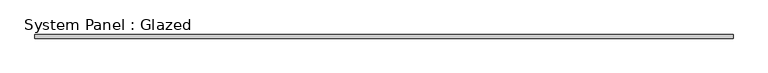
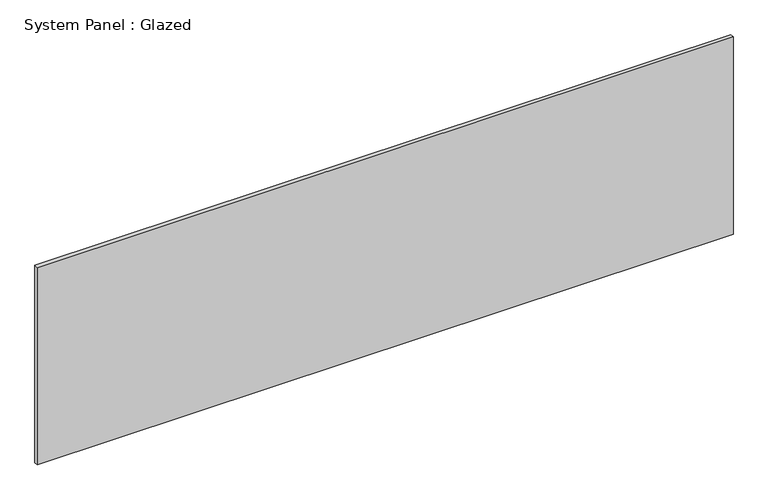
"""IFC4 building model written with IfcOpenShell, lengths in millimetres: plate geometry, System Panel : Glazed."""

from ifc_helpers import new_model, si_unit, origin, origin_with_axes, place, context, project, spatial, polyline, outline, extrude, source, transform, mapped, element, save


def system_panel_glazed_242742f8(model_context):
    return source(origin(), model_context, "Body", "SweptSolid", [
        extrude(outline(polyline([(2438.4, 19.05), (-2438.4, 19.05), (-2438.4, 44.45), (2438.4, 44.45), (2438.4, 19.05)])), origin_with_axes(), (0.0, 0.0, 1.0), 1460.5),
    ])


if __name__ == "__main__":
    model = new_model("IFC4")
    model_context = context("Model", 3, world=origin())
    ifc_project = project(units=[si_unit("LENGTHUNIT", "METRE", prefix="MILLI")], contexts=[model_context])
    site = spatial("IfcSite", under=ifc_project)
    building = spatial("IfcBuilding", under=site)
    placement = place(None, origin())
    system_panel_glazed_shape = system_panel_glazed_242742f8(model_context)
    element("IfcPlate", 1, ObjectType="System Panel : Glazed", at=placement, inside=building, context=model_context, shape_type="MappedRepresentation", body=[
        mapped(system_panel_glazed_shape, transform((0.0, 0.0, 0.0), x_axis=(1.0, 0.0, 0.0), y_axis=(0.0, 1.0, 0.0), z_axis=(0.0, 0.0, 1.0))),
    ])
    save(model, "model.ifc")

# Revit data of these elements
# Type "System Panel : Glazed"
#   Construction Type Id = "GSP4R"
#   Analytic Construction = "1/8 in Pilkington single glazing"
#   Visual Light Transmittance = 0.9
#   Solar Heat Gain Coefficient = 0.86
#   Heat Transfer Coefficient (U) = 1.18115 BTU/(h·ft²·°F)
# Element 1 (IfcPlate, "System Panel : Glazed")
#   Materials on its faces: "Glass"
# Materials
#   "Glass": class "Glass", colour RGB 0 128 192, transparency 0.75, Description = "Soda Lime Glass", Cost = 0
